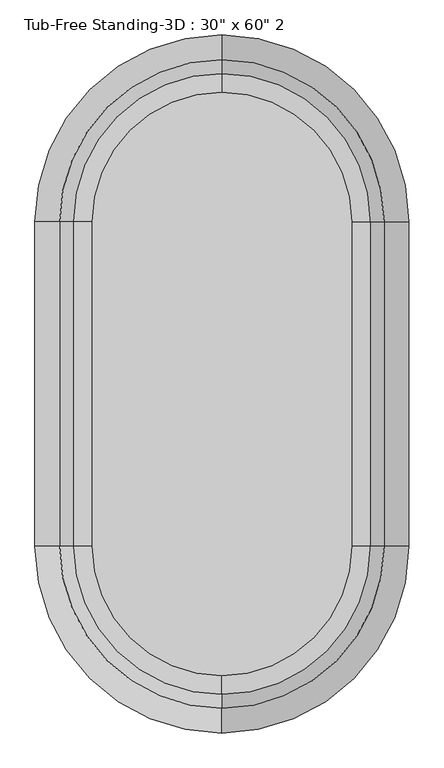
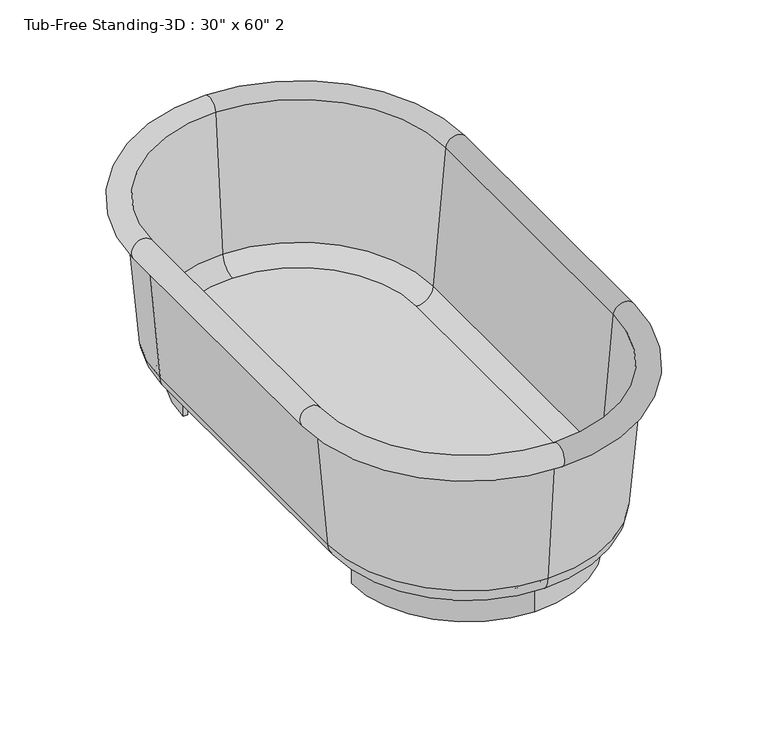
"""IFC4 building model written with IfcOpenShell, lengths in millimetres: flow terminal geometry."""

from ifc_helpers import new_model, si_unit, point, frame, frame_2d, origin, origin_with_axes, place, context, project, spatial, polyline, circle_curve, ellipse_curve, trimmed, segment, composite_curve, outline, extrude, source, transform, mapped, element, save
from ifc_brep_helpers import plane_surface, cylinder_surface, revolved_surface, advanced_brep


def flow_terminal_a2f06f5b(model_context):
    return source(origin(), model_context, "Body", "SolidModel", [
        extrude(outline(composite_curve([segment(trimmed(circle_curve(frame_2d((0.0, 330.2)), 254.0), [point((0.0, 584.2))], [point((-254.0, 330.2))], True, "CARTESIAN"), True, "CONTINUOUS"), segment(polyline([(-254.0, 330.2), (-264.2824236, 330.2)]), True, "CONTINUOUS"), segment(trimmed(circle_curve(frame_2d((0.0, 330.2)), 264.2824236), [point((-264.2824236, 330.2))], [point((0.0, 594.4824236))], False, "CARTESIAN"), True, "CONTINUOUS"), segment(trimmed(circle_curve(frame_2d((0.0, 330.2)), 264.2824236), [point((0.0, 594.4824236))], [point((264.2824236, 330.2))], False, "CARTESIAN"), True, "CONTINUOUS"), segment(polyline([(264.2824236, 330.2), (254.0, 330.2)]), True, "CONTINUOUS"), segment(trimmed(circle_curve(frame_2d((0.0, 330.2)), 254.0), [point((254.0, 330.2))], [point((0.0, 584.2))], True, "CARTESIAN"), True, "CONTINUOUS")], self_intersect=False)), origin_with_axes(), (0.0, 0.0, 1.0), 63.5),
        extrude(outline(composite_curve([segment(trimmed(circle_curve(frame_2d((0.0, -330.2)), 264.2824236), [point((0.0, -594.4824236))], [point((-264.2824236, -330.2))], False, "CARTESIAN"), True, "CONTINUOUS"), segment(polyline([(-264.2824236, -330.2), (-254.0, -330.2)]), True, "CONTINUOUS"), segment(trimmed(circle_curve(frame_2d((0.0, -330.2)), 254.0), [point((-254.0, -330.2))], [point((0.0, -584.2))], True, "CARTESIAN"), True, "CONTINUOUS"), segment(trimmed(circle_curve(frame_2d((0.0, -330.2)), 254.0), [point((0.0, -584.2))], [point((254.0, -330.2))], True, "CARTESIAN"), True, "CONTINUOUS"), segment(polyline([(254.0, -330.2), (264.2824236, -330.2)]), True, "CONTINUOUS"), segment(trimmed(circle_curve(frame_2d((0.0, -330.2)), 264.2824236), [point((264.2824236, -330.2))], [point((0.0, -594.4824236))], False, "CARTESIAN"), True, "CONTINUOUS")], self_intersect=False)), origin_with_axes(), (0.0, 0.0, 1.0), 63.5),
        extrude(outline(composite_curve([segment(polyline([(-264.2824236, -330.2), (-264.2824236, 330.2)]), True, "CONTINUOUS"), segment(trimmed(circle_curve(frame_2d((0.0, 330.2)), 264.2824236), [point((-264.2824236, 330.2))], [point((0.0, 594.4824236))], False, "CARTESIAN"), True, "CONTINUOUS"), segment(trimmed(circle_curve(frame_2d((0.0, 330.2)), 264.2824236), [point((0.0, 594.4824236))], [point((264.2824236, 330.2))], False, "CARTESIAN"), True, "CONTINUOUS"), segment(polyline([(264.2824236, 330.2), (264.2824236, -330.2)]), True, "CONTINUOUS"), segment(trimmed(circle_curve(frame_2d((0.0, -330.2)), 264.2824236), [point((264.2824236, -330.2))], [point((0.0, -594.4824236))], False, "CARTESIAN"), True, "CONTINUOUS"), segment(trimmed(circle_curve(frame_2d((0.0, -330.2)), 264.2824236), [point((0.0, -594.4824236))], [point((-264.2824236, -330.2))], False, "CARTESIAN"), True, "CONTINUOUS")], self_intersect=False)), frame((0.0, 0.0, 63.5), z_axis=(0.0, 0.0, 1.0), x_axis=(1.0, 0.0, 0.0)), (0.0, 0.0, 1.0), 15.08125),
        advanced_brep(
        [(0.0, -673.1, 406.4), (342.9, -330.2, 406.4), (355.6, -330.2, 406.4), (0.0, -685.8, 406.4), (0.0, -647.3045038, 111.5561295), (317.1045038, -330.2, 111.5561295), (0.0, -594.4824236, 63.1536107), (264.2824236, -330.2, 63.1536107), (0.0, -594.4824236, 78.0774627), (264.2824236, -330.2, 78.0774627), (0.0, -632.4374416, 112.8568289), (302.2374416, -330.2, 112.8568289), (0.0, -660.6561556, 435.3982063), (330.4561556, -330.2, 435.3982063), (-342.9, -330.2, 406.4), (-355.6, -330.2, 406.4), (-317.1045038, -330.2, 111.5561295), (-264.2824236, -330.2, 63.1536107), (-264.2824236, -330.2, 78.0774627), (-302.2374416, -330.2, 112.8568289), (-330.4561556, -330.2, 435.3982063), (-355.6, 330.2, 406.4), (-342.9, 330.2, 406.4), (-317.1045038, 330.2, 111.5561295), (-264.2824236, 330.2, 63.1536107), (-264.2824236, 330.2, 78.0774627), (-302.2374416, 330.2, 112.8568289), (-330.4561556, 330.2, 435.3982063), (0.0, 673.1, 406.4), (0.0, 685.8, 406.4), (0.0, 647.3045038, 111.5561295), (0.0, 594.4824236, 63.1536107), (0.0, 594.4824236, 78.0774627), (0.0, 632.4374416, 112.8568289), (0.0, 660.6561556, 435.3982063), (342.9, 330.2, 406.4), (355.6, 330.2, 406.4), (317.1045038, 330.2, 111.5561295), (264.2824236, 330.2, 63.1536107), (264.2824236, 330.2, 78.0774627), (302.2374416, 330.2, 112.8568289), (330.4561556, 330.2, 435.3982063)],
        [
            (0, 1, circle_curve(frame((0.0, -330.2, 406.4), z_axis=(0.0, 0.0, 1.0), x_axis=(1.0, 0.0, 0.0)), 342.9)),
            (1, 2),
            (2, 3, circle_curve(frame((0.0, -330.2, 406.4), z_axis=(0.0, 0.0, -1.0), x_axis=(1.0, 0.0, 0.0)), 355.6)),
            (3, 0),
            (4, 5, circle_curve(frame((0.0, -330.2, 111.5561295), z_axis=(0.0, 0.0, 1.0), x_axis=(1.0, 0.0, 0.0)), 317.1045038)),
            (5, 1),
            (0, 4),
            (6, 7, circle_curve(frame((0.0, -330.2, 63.1536107), z_axis=(0.0, 0.0, 1.0), x_axis=(1.0, 0.0, 0.0)), 264.2824236)),
            (7, 5, circle_curve(frame((264.2824236, -330.2, 116.1774627), z_axis=(0.0, -1.0, 0.0), x_axis=(1.0, 0.0, 0.0)), 53.023852)),
            (4, 6, circle_curve(frame((0.0, -594.4824236, 116.1774627), z_axis=(1.0, 0.0, 0.0), x_axis=(0.0, -1.0, 0.0)), 53.023852)),
            (8, 9, circle_curve(frame((0.0, -330.2, 78.0774627), z_axis=(0.0, 0.0, 1.0), x_axis=(1.0, 0.0, 0.0)), 264.2824236)),
            (9, 7),
            (6, 8),
            (10, 11, circle_curve(frame((0.0, -330.2, 112.8568289), z_axis=(0.0, 0.0, 1.0), x_axis=(1.0, 0.0, 0.0)), 302.2374416)),
            (11, 9, circle_curve(frame((264.2824236, -330.2, 116.1774627), z_axis=(0.0, 1.0, 0.0), x_axis=(1.0, 0.0, 0.0)), 38.1)),
            (8, 10, circle_curve(frame((0.0, -594.4824236, 116.1774627), z_axis=(-1.0, 0.0, 0.0), x_axis=(0.0, -1.0, 0.0)), 38.1)),
            (12, 13, circle_curve(frame((0.0, -330.2, 435.3982063), z_axis=(0.0, 0.0, 1.0), x_axis=(1.0, 0.0, 0.0)), 330.4561556)),
            (13, 11),
            (10, 12),
            (2, 13, circle_curve(frame((355.6, -330.2, 431.8), z_axis=(0.0, -1.0, 0.0), x_axis=(1.0, 0.0, 0.0)), 25.4)),
            (12, 3, circle_curve(frame((0.0, -685.8, 431.8), z_axis=(1.0, 0.0, 0.0), x_axis=(0.0, -1.0, 0.0)), 25.4)),
            (14, 0, circle_curve(frame((0.0, -330.2, 406.4), z_axis=(0.0, 0.0, 1.0), x_axis=(0.0, -1.0, 0.0)), 342.9)),
            (3, 15, circle_curve(frame((0.0, -330.2, 406.4), z_axis=(0.0, 0.0, -1.0), x_axis=(0.0, -1.0, 0.0)), 355.6)),
            (15, 14),
            (16, 4, circle_curve(frame((0.0, -330.2, 111.5561295), z_axis=(0.0, 0.0, 1.0), x_axis=(0.0, -1.0, 0.0)), 317.1045038)),
            (14, 16),
            (17, 6, circle_curve(frame((0.0, -330.2, 63.1536107), z_axis=(0.0, 0.0, 1.0), x_axis=(0.0, -1.0, 0.0)), 264.2824236)),
            (16, 17, circle_curve(frame((-264.2824236, -330.2, 116.1774627), z_axis=(0.0, -1.0, 0.0), x_axis=(-1.0, 0.0, 0.0)), 53.023852)),
            (18, 8, circle_curve(frame((0.0, -330.2, 78.0774627), z_axis=(0.0, 0.0, 1.0), x_axis=(0.0, -1.0, 0.0)), 264.2824236)),
            (17, 18),
            (19, 10, circle_curve(frame((0.0, -330.2, 112.8568289), z_axis=(0.0, 0.0, 1.0), x_axis=(0.0, -1.0, 0.0)), 302.2374416)),
            (18, 19, circle_curve(frame((-264.2824236, -330.2, 116.1774627), z_axis=(0.0, 1.0, 0.0), x_axis=(-1.0, 0.0, 0.0)), 38.1)),
            (20, 12, circle_curve(frame((0.0, -330.2, 435.3982063), z_axis=(0.0, 0.0, 1.0), x_axis=(0.0, -1.0, 0.0)), 330.4561556)),
            (19, 20),
            (20, 15, circle_curve(frame((-355.6, -330.2, 431.8), z_axis=(0.0, -1.0, 0.0), x_axis=(-1.0, 0.0, 0.0)), 25.4)),
            (15, 21),
            (21, 22),
            (22, 14),
            (22, 23),
            (23, 16),
            (23, 24, circle_curve(frame((-264.2824236, 330.2, 116.1774627), z_axis=(0.0, -1.0, 0.0), x_axis=(-1.0, 0.0, 0.0)), 53.023852)),
            (24, 17),
            (24, 25),
            (25, 18),
            (25, 26, circle_curve(frame((-264.2824236, 330.2, 116.1774627), z_axis=(0.0, 1.0, 0.0), x_axis=(-1.0, 0.0, 0.0)), 38.1)),
            (26, 19),
            (26, 27),
            (27, 20),
            (27, 21, circle_curve(frame((-355.6, 330.2, 431.8), z_axis=(0.0, -1.0, 0.0), x_axis=(-1.0, 0.0, 0.0)), 25.4)),
            (28, 22, circle_curve(frame((0.0, 330.2, 406.4), z_axis=(0.0, 0.0, 1.0), x_axis=(-1.0, 0.0, 0.0)), 342.9)),
            (21, 29, circle_curve(frame((0.0, 330.2, 406.4), z_axis=(0.0, 0.0, -1.0), x_axis=(-1.0, 0.0, 0.0)), 355.6)),
            (29, 28),
            (30, 23, circle_curve(frame((0.0, 330.2, 111.5561295), z_axis=(0.0, 0.0, 1.0), x_axis=(-1.0, 0.0, 0.0)), 317.1045038)),
            (28, 30),
            (31, 24, circle_curve(frame((0.0, 330.2, 63.1536107), z_axis=(0.0, 0.0, 1.0), x_axis=(-1.0, 0.0, 0.0)), 264.2824236)),
            (30, 31, circle_curve(frame((0.0, 594.4824236, 116.1774627), z_axis=(-1.0, 0.0, 0.0), x_axis=(0.0, 1.0, 0.0)), 53.023852)),
            (32, 25, circle_curve(frame((0.0, 330.2, 78.0774627), z_axis=(0.0, 0.0, 1.0), x_axis=(-1.0, 0.0, 0.0)), 264.2824236)),
            (31, 32),
            (33, 26, circle_curve(frame((0.0, 330.2, 112.8568289), z_axis=(0.0, 0.0, 1.0), x_axis=(-1.0, 0.0, 0.0)), 302.2374416)),
            (32, 33, circle_curve(frame((0.0, 594.4824236, 116.1774627), z_axis=(1.0, 0.0, 0.0), x_axis=(0.0, 1.0, 0.0)), 38.1)),
            (34, 27, circle_curve(frame((0.0, 330.2, 435.3982063), z_axis=(0.0, 0.0, 1.0), x_axis=(-1.0, 0.0, 0.0)), 330.4561556)),
            (33, 34),
            (34, 29, circle_curve(frame((0.0, 685.8, 431.8), z_axis=(-1.0, 0.0, 0.0), x_axis=(0.0, 1.0, 0.0)), 25.4)),
            (35, 28, circle_curve(frame((0.0, 330.2, 406.4), z_axis=(0.0, 0.0, 1.0), x_axis=(0.0, 1.0, 0.0)), 342.9)),
            (29, 36, circle_curve(frame((0.0, 330.2, 406.4), z_axis=(0.0, 0.0, -1.0), x_axis=(0.0, 1.0, 0.0)), 355.6)),
            (36, 35),
            (37, 30, circle_curve(frame((0.0, 330.2, 111.5561295), z_axis=(0.0, 0.0, 1.0), x_axis=(0.0, 1.0, 0.0)), 317.1045038)),
            (35, 37),
            (38, 31, circle_curve(frame((0.0, 330.2, 63.1536107), z_axis=(0.0, 0.0, 1.0), x_axis=(0.0, 1.0, 0.0)), 264.2824236)),
            (37, 38, circle_curve(frame((264.2824236, 330.2, 116.1774627), z_axis=(0.0, 1.0, 0.0), x_axis=(1.0, 0.0, 0.0)), 53.023852)),
            (39, 32, circle_curve(frame((0.0, 330.2, 78.0774627), z_axis=(0.0, 0.0, 1.0), x_axis=(0.0, 1.0, 0.0)), 264.2824236)),
            (38, 39),
            (40, 33, circle_curve(frame((0.0, 330.2, 112.8568289), z_axis=(0.0, 0.0, 1.0), x_axis=(0.0, 1.0, 0.0)), 302.2374416)),
            (39, 40, circle_curve(frame((264.2824236, 330.2, 116.1774627), z_axis=(0.0, -1.0, 0.0), x_axis=(1.0, 0.0, 0.0)), 38.1)),
            (41, 34, circle_curve(frame((0.0, 330.2, 435.3982063), z_axis=(0.0, 0.0, 1.0), x_axis=(0.0, 1.0, 0.0)), 330.4561556)),
            (40, 41),
            (41, 36, circle_curve(frame((355.6, 330.2, 431.8), z_axis=(0.0, 1.0, 0.0), x_axis=(1.0, 0.0, 0.0)), 25.4)),
            (36, 2),
            (1, 35),
            (5, 37),
            (7, 38),
            (9, 39),
            (11, 40),
            (13, 41),
        ],
        [
            plane_surface(frame((0.0, -330.2, 406.4), z_axis=(0.0, 0.0, -1.0), x_axis=(1.0, 0.0, 0.0))),
            revolved_surface(polyline([(342.9, -330.2, 406.4), (317.1045038, -330.2, 111.5561295)]), (0.0, -330.2, 431.8), (0.0, 0.0, -1.0)),
            revolved_surface(trimmed(ellipse_curve(frame((264.2824236, -330.2, 116.1774627), z_axis=(0.0, 1.0, 0.0), x_axis=(1.0, 0.0, 0.0)), 53.023852, 53.023852), [point((317.1045038, -330.2, 111.5561295))], [point((264.2824236, -330.2, 63.1536107))], True, "CARTESIAN"), (0.0, -330.2, 431.8), (0.0, 0.0, -1.0)),
            revolved_surface(polyline([(264.2824236, -330.2, 63.1536107), (264.2824236, -330.2, 78.07746270000001)]), (0.0, -330.2, 431.8), (0.0, 0.0, -1.0)),
            revolved_surface(trimmed(ellipse_curve(frame((264.2824236, -330.2, 116.1774627), z_axis=(0.0, -1.0, 0.0), x_axis=(1.0, 0.0, 0.0)), 38.1, 38.1), [point((264.2824236, -330.2, 78.0774627))], [point((302.2374416, -330.2, 112.8568289))], True, "CARTESIAN"), (0.0, -330.2, 431.8), (0.0, 0.0, -1.0)),
            revolved_surface(polyline([(302.2374416, -330.2, 112.8568289), (330.4561556, -330.2, 435.3982063)]), (0.0, -330.2, 431.8), (0.0, 0.0, -1.0)),
            revolved_surface(trimmed(ellipse_curve(frame((355.6, -330.2, 431.8), z_axis=(0.0, 1.0, 0.0), x_axis=(1.0, 0.0, 0.0)), 25.4, 25.4), [point((330.4561556, -330.2, 435.3982063))], [point((355.6, -330.2, 406.4))], True, "CARTESIAN"), (0.0, -330.2, 431.8), (0.0, 0.0, -1.0)),
            plane_surface(frame((0.0, -330.2, 406.4), z_axis=(0.0, 0.0, -1.0), x_axis=(0.0, -1.0, 0.0))),
            revolved_surface(polyline([(0.0, -673.1, 406.4), (0.0, -647.3045038, 111.5561295)]), (0.0, -330.2, 431.8), (0.0, 0.0, -1.0)),
            revolved_surface(trimmed(ellipse_curve(frame((0.0, -594.4824236, 116.1774627), z_axis=(1.0, 0.0, 0.0), x_axis=(0.0, -1.0, 0.0)), 53.023852, 53.023852), [point((0.0, -647.3045038, 111.5561295))], [point((0.0, -594.4824236, 63.1536107))], True, "CARTESIAN"), (0.0, -330.2, 431.8), (0.0, 0.0, -1.0)),
            revolved_surface(polyline([(0.0, -594.4824236, 63.1536107), (0.0, -594.4824236, 78.07746270000001)]), (0.0, -330.2, 431.8), (0.0, 0.0, -1.0)),
            revolved_surface(trimmed(ellipse_curve(frame((0.0, -594.4824236, 116.1774627), z_axis=(-1.0, 0.0, 0.0), x_axis=(0.0, -1.0, 0.0)), 38.1, 38.1), [point((0.0, -594.4824236, 78.0774627))], [point((0.0, -632.4374416, 112.8568289))], True, "CARTESIAN"), (0.0, -330.2, 431.8), (0.0, 0.0, -1.0)),
            revolved_surface(polyline([(0.0, -632.4374416, 112.8568289), (0.0, -660.6561556, 435.3982063)]), (0.0, -330.2, 431.8), (0.0, 0.0, -1.0)),
            revolved_surface(trimmed(ellipse_curve(frame((0.0, -685.8, 431.8), z_axis=(1.0, 0.0, 0.0), x_axis=(0.0, -1.0, 0.0)), 25.4, 25.4), [point((0.0, -660.6561556, 435.3982063))], [point((0.0, -685.8, 406.4))], True, "CARTESIAN"), (0.0, -330.2, 431.8), (0.0, 0.0, -1.0)),
            plane_surface(frame((-355.6, -330.2, 406.4), z_axis=(0.0, 0.0, -1.0), x_axis=(0.0, 1.0, 0.0))),
            plane_surface(frame((-342.9, -330.2, 406.4), z_axis=(-0.9961946980917455, 0.0, -0.08715574274765871), x_axis=(0.0, 1.0, 0.0))),
            cylinder_surface(frame((-264.2824236, -330.2, 116.1774627), z_axis=(0.0, -1.0, 0.0), x_axis=(-1.0, 0.0, 0.0)), 53.023852),
            plane_surface(frame((-264.2824236, -330.2, 63.1536107), z_axis=(1.0, 0.0, 0.0), x_axis=(0.0, 1.0, 0.0))),
            revolved_surface(polyline([(-302.38242360000004, 330.2, 116.1774627), (-302.38242360000004, -330.2, 116.1774627)]), (-264.2824236, -330.2, 116.1774627), (0.0, 1.0, 0.0)),
            plane_surface(frame((-302.2374416, -330.2, 112.8568289), z_axis=(0.9961946980917458, 0.0, 0.08715574274765651), x_axis=(0.0, 1.0, 0.0))),
            cylinder_surface(frame((-355.6, -330.2, 431.8), z_axis=(0.0, -1.0, 0.0), x_axis=(-1.0, 0.0, 0.0)), 25.4),
            plane_surface(frame((0.0, 330.2, 406.4), z_axis=(0.0, 0.0, -1.0), x_axis=(-1.0, 0.0, 0.0))),
            revolved_surface(polyline([(-342.9, 330.2, 406.4), (-317.1045038, 330.2, 111.5561295)]), (0.0, 330.2, 431.8), (0.0, 0.0, -1.0)),
            revolved_surface(trimmed(ellipse_curve(frame((-264.2824236, 330.2, 116.1774627), z_axis=(0.0, -1.0, 0.0), x_axis=(-1.0, 0.0, 0.0)), 53.023852, 53.023852), [point((-317.1045038, 330.2, 111.5561295))], [point((-264.2824236, 330.2, 63.1536107))], True, "CARTESIAN"), (0.0, 330.2, 431.8), (0.0, 0.0, -1.0)),
            revolved_surface(polyline([(-264.2824236, 330.2, 63.1536107), (-264.2824236, 330.2, 78.07746270000001)]), (0.0, 330.2, 431.8), (0.0, 0.0, -1.0)),
            revolved_surface(trimmed(ellipse_curve(frame((-264.2824236, 330.2, 116.1774627), z_axis=(0.0, 1.0, 0.0), x_axis=(-1.0, 0.0, 0.0)), 38.1, 38.1), [point((-264.2824236, 330.2, 78.0774627))], [point((-302.2374416, 330.2, 112.8568289))], True, "CARTESIAN"), (0.0, 330.2, 431.8), (0.0, 0.0, -1.0)),
            revolved_surface(polyline([(-302.2374416, 330.2, 112.8568289), (-330.4561556, 330.2, 435.3982063)]), (0.0, 330.2, 431.8), (0.0, 0.0, -1.0)),
            revolved_surface(trimmed(ellipse_curve(frame((-355.6, 330.2, 431.8), z_axis=(0.0, -1.0, 0.0), x_axis=(-1.0, 0.0, 0.0)), 25.4, 25.4), [point((-330.4561556, 330.2, 435.3982063))], [point((-355.6, 330.2, 406.4))], True, "CARTESIAN"), (0.0, 330.2, 431.8), (0.0, 0.0, -1.0)),
            plane_surface(frame((0.0, 330.2, 406.4), z_axis=(0.0, 0.0, -1.0), x_axis=(0.0, 1.0, 0.0))),
            revolved_surface(polyline([(0.0, 673.1, 406.4), (0.0, 647.3045038, 111.5561295)]), (0.0, 330.2, 431.8), (0.0, 0.0, -1.0)),
            revolved_surface(trimmed(ellipse_curve(frame((0.0, 594.4824236, 116.1774627), z_axis=(-1.0, 0.0, 0.0), x_axis=(0.0, 1.0, 0.0)), 53.023852, 53.023852), [point((0.0, 647.3045038, 111.5561295))], [point((0.0, 594.4824236, 63.1536107))], True, "CARTESIAN"), (0.0, 330.2, 431.8), (0.0, 0.0, -1.0)),
            revolved_surface(polyline([(0.0, 594.4824236, 63.1536107), (0.0, 594.4824236, 78.07746270000001)]), (0.0, 330.2, 431.8), (0.0, 0.0, -1.0)),
            revolved_surface(trimmed(ellipse_curve(frame((0.0, 594.4824236, 116.1774627), z_axis=(1.0, 0.0, 0.0), x_axis=(0.0, 1.0, 0.0)), 38.1, 38.1), [point((0.0, 594.4824236, 78.0774627))], [point((0.0, 632.4374416, 112.8568289))], True, "CARTESIAN"), (0.0, 330.2, 431.8), (0.0, 0.0, -1.0)),
            revolved_surface(polyline([(0.0, 632.4374416, 112.8568289), (0.0, 660.6561556, 435.3982063)]), (0.0, 330.2, 431.8), (0.0, 0.0, -1.0)),
            revolved_surface(trimmed(ellipse_curve(frame((0.0, 685.8, 431.8), z_axis=(-1.0, 0.0, 0.0), x_axis=(0.0, 1.0, 0.0)), 25.4, 25.4), [point((0.0, 660.6561556, 435.3982063))], [point((0.0, 685.8, 406.4))], True, "CARTESIAN"), (0.0, 330.2, 431.8), (0.0, 0.0, -1.0)),
            plane_surface(frame((355.6, 330.2, 406.4), z_axis=(0.0, 0.0, -1.0), x_axis=(0.0, -1.0, 0.0))),
            plane_surface(frame((342.9, 330.2, 406.4), z_axis=(0.9961946980917455, 0.0, -0.08715574274765871), x_axis=(0.0, -1.0, 0.0))),
            cylinder_surface(frame((264.2824236, 330.2, 116.1774627), z_axis=(0.0, 1.0, 0.0), x_axis=(1.0, 0.0, 0.0)), 53.023852),
            plane_surface(frame((264.2824236, 330.2, 63.1536107), z_axis=(-1.0, 0.0, 0.0), x_axis=(0.0, -1.0, 0.0))),
            revolved_surface(polyline([(302.38242360000004, -330.2, 116.1774627), (302.38242360000004, 330.2, 116.1774627)]), (264.2824236, 330.2, 116.1774627), (0.0, -1.0, 0.0)),
            plane_surface(frame((302.2374416, 330.2, 112.8568289), z_axis=(-0.9961946980917458, 0.0, 0.08715574274765651), x_axis=(0.0, -1.0, 0.0))),
            cylinder_surface(frame((355.6, 330.2, 431.8), z_axis=(0.0, 1.0, 0.0), x_axis=(1.0, 0.0, 0.0)), 25.4),
        ],
        [
            (0, [[1, 2, 3, 4]]),
            (1, [[5, 6, -1, 7]]),
            (2, [[8, 9, -5, 10]]),
            (3, [[11, 12, -8, 13]]),
            (4, [[14, 15, -11, 16]]),
            (5, [[17, 18, -14, 19]]),
            (6, [[-3, 20, -17, 21]]),
            (7, [[22, -4, 23, 24]]),
            (8, [[25, -7, -22, 26]]),
            (9, [[27, -10, -25, 28]]),
            (10, [[29, -13, -27, 30]]),
            (11, [[31, -16, -29, 32]]),
            (12, [[33, -19, -31, 34]]),
            (13, [[-23, -21, -33, 35]]),
            (14, [[-24, 36, 37, 38]]),
            (15, [[-26, -38, 39, 40]]),
            (16, [[-28, -40, 41, 42]]),
            (17, [[-30, -42, 43, 44]]),
            (18, [[-32, -44, 45, 46]]),
            (19, [[-34, -46, 47, 48]]),
            (20, [[-35, -48, 49, -36]]),
            (21, [[50, -37, 51, 52]]),
            (22, [[53, -39, -50, 54]]),
            (23, [[55, -41, -53, 56]]),
            (24, [[57, -43, -55, 58]]),
            (25, [[59, -45, -57, 60]]),
            (26, [[61, -47, -59, 62]]),
            (27, [[-51, -49, -61, 63]]),
            (28, [[64, -52, 65, 66]]),
            (29, [[67, -54, -64, 68]]),
            (30, [[69, -56, -67, 70]]),
            (31, [[71, -58, -69, 72]]),
            (32, [[73, -60, -71, 74]]),
            (33, [[75, -62, -73, 76]]),
            (34, [[-65, -63, -75, 77]]),
            (35, [[-66, 78, -2, 79]]),
            (36, [[-68, -79, -6, 80]]),
            (37, [[-70, -80, -9, 81]]),
            (38, [[-72, -81, -12, 82]]),
            (39, [[-74, -82, -15, 83]]),
            (40, [[-76, -83, -18, 84]]),
            (41, [[-77, -84, -20, -78]]),
        ],
    ),
    ])


if __name__ == "__main__":
    model = new_model("IFC4")
    model_context = context("Model", 3, world=origin())
    ifc_project = project(units=[si_unit("LENGTHUNIT", "METRE", prefix="MILLI")], contexts=[model_context])
    site = spatial("IfcSite", under=ifc_project)
    building = spatial("IfcBuilding", under=site)
    placement = place(None, origin())
    flow_terminal_shape = flow_terminal_a2f06f5b(model_context)
    element("IfcFlowTerminal", 1, ObjectType="Tub-Free Standing-3D : 30\" x 60\" 2", at=placement, inside=building, context=model_context, shape_type="MappedRepresentation", body=[
        mapped(flow_terminal_shape, transform((0.0, 0.0, 0.0), x_axis=(1.0, 0.0, 0.0), y_axis=(0.0, 1.0, 0.0), z_axis=(0.0, 0.0, 1.0))),
    ])
    save(model, "model.ifc")

# Revit data of these elements
# Type "Tub-Free Standing-3D : 30\" x 60\" 2"
#   Assembly Code = "D2010110"
#   Height = 1' - 6"
#   Length = 4' - 8"
#   Width = 2' - 6"
#   Tub Material = Porcelain, Ivory
#   Default Elevation = 0
# Element 1 (IfcFlowTerminal, "Tub-Free Standing-3D : 30\" x 60\" 2")
#   Materials on its faces: "Porcelain, Ivory"
# Materials
#   "Porcelain, Ivory": class "Ceramic", colour RGB 247 247 239, transparency 0, Description = "Porcelain, ivory", Cost = 0
